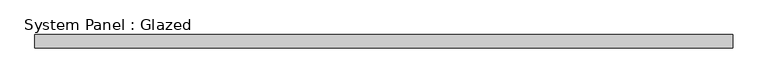
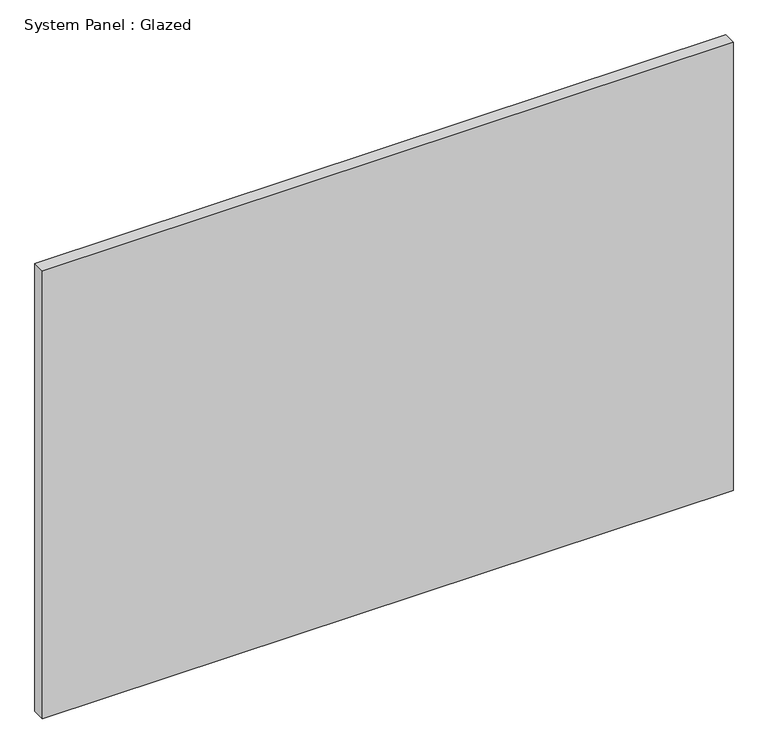
"""IFC4 building model written with IfcOpenShell, lengths in millimetres: plate geometry, System Panel : Glazed."""

from ifc_helpers import new_model, si_unit, origin, origin_with_axes, place, context, project, spatial, polyline, outline, extrude, source, transform, mapped, element, save


def system_panel_glazed_6c2f0e29(model_context):
    return source(origin(), model_context, "Body", "SweptSolid", [
        extrude(outline(polyline([(670.9833332, 19.05), (-670.9833332, 19.05), (-670.9833332, 44.45), (670.9833332, 44.45), (670.9833332, 19.05)])), origin_with_axes(), (0.0, 0.0, 1.0), 920.75),
    ])


if __name__ == "__main__":
    model = new_model("IFC4")
    model_context = context("Model", 3, world=origin())
    ifc_project = project(units=[si_unit("LENGTHUNIT", "METRE", prefix="MILLI")], contexts=[model_context])
    site = spatial("IfcSite", under=ifc_project)
    building = spatial("IfcBuilding", under=site)
    placement = place(None, origin())
    system_panel_glazed_shape = system_panel_glazed_6c2f0e29(model_context)
    element("IfcPlate", 1, ObjectType="System Panel : Glazed", at=placement, inside=building, context=model_context, shape_type="MappedRepresentation", body=[
        mapped(system_panel_glazed_shape, transform((0.0, 0.0, 0.0), x_axis=(1.0, 0.0, 0.0), y_axis=(0.0, 1.0, 0.0), z_axis=(0.0, 0.0, 1.0))),
    ])
    save(model, "model.ifc")

# Revit data of these elements
# Type "System Panel : Glazed"
#   Construction Type Id = "GSP4R"
#   Analytic Construction = "1/8 in Pilkington single glazing"
#   Visual Light Transmittance = 0.9
#   Solar Heat Gain Coefficient = 0.86
#   Heat Transfer Coefficient (U) = 1.18115 BTU/(h·ft²·°F)
#   Define Thermal Properties by = 1
# Element 1 (IfcPlate, "System Panel : Glazed")
#   Materials on its faces: "glass panel 223"
# Materials
#   "glass panel 223": class "Generic", colour RGB 120 120 120, transparency 0, Cost = 0
